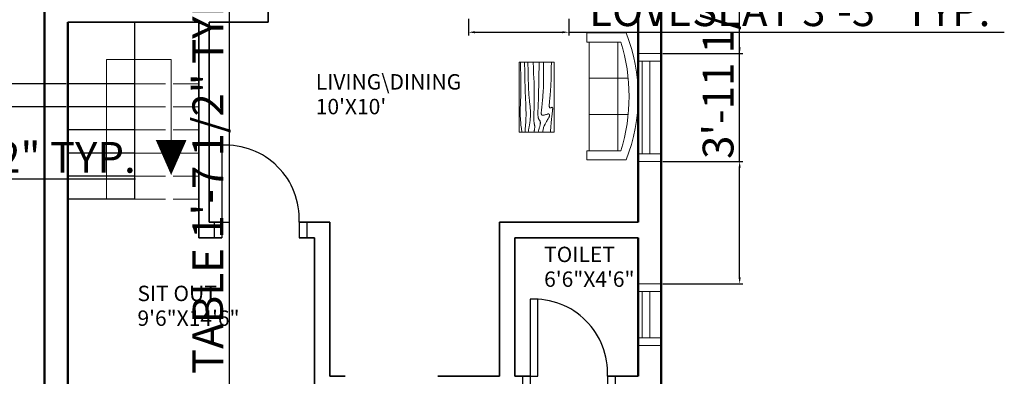
# Model space of a CAD drawing. Units: inches. Extents: x 2296 to 3335, y 495 to 1294.
# Tile 6 of 7: x 2952 to 3335, y 723 to 862. Entities that reach past the tile are written whole.
import ezdxf

# ---------------------------------------------------------------- set-up
doc = ezdxf.new("R2010")
doc.units = ezdxf.units.IN
doc.linetypes.add('ACAD_ISO02W100', pattern=[15, 12, -3])
for name, color, linetype, lineweight in [('A-ANNO-DIMS', 2, 'Continuous', 18), ('A-ANNO-SYMB', 7, 'Continuous', 18), ('A-AREA-IDEN', 7, 'Continuous', 18), ('A-FLOR-STRS', 7, 'Continuous', 25), ('A-FLOR-STRS-OVHD', 7, 'ACAD_ISO02W100', 18), ('DOORS', 1, 'Continuous', 25), ('FURNITURE', 2, 'Continuous', 18), ('INNER WALL', 6, 'Continuous', 35), ('OUTER WALL', 5, 'Continuous', 50), ('VENTILATOR', 4, 'Continuous', 18), ('WINDOWS', 3, 'Continuous', 18)]:
    doc.layers.add(name, color=color, linetype=linetype, lineweight=lineweight)
doc.styles.get("Standard").update_dxf_attribs({"font": 'arial.ttf'})
doc.dimstyles.new('ISO-25', dxfattribs={"dimtxt": 12, "dimasz": 2.5, "dimexe": 1.25, "dimexo": 0.625, "dimtad": 1, "dimdec": 1, "dimlunit": 3, "dimtxsty": 'Standard', "dimcen": 2.5, "dimadec": 0, "dimazin": 0, "dimtfac": 1, "dimtdec": 1, "dimtmove": 0, "dimatfit": 3, "dimfxl": 1, "dimarcsym": 0})

# ---------------------------------------------------------------- blocks, each defined once
blk = doc.blocks.new('Sofa - Roundback 7 ft.')
for p, q in [((-36.000027, -34), (-36.000027, -11.4696)), ((-12.00002, -32.4421), (-12.00003, -6.5971)), ((11.99997, -32.4421), (11.99998, -6.5971)), ((35.99998, -34), (35.99998, -11.4696)), ((-35.999844, -13.3819), (35.9998, -13.3819)), ((-36.000027, -32.4421), (35.99998, -32.4421))]:
    blk.add_line(p, q)
for points in [[(-36.000027, -34), (-42.000027, -34), (-42.000027, -8)], [(41.99998, -8), (41.99998, -34), (35.99998, -34)]]:
    blk.add_lwpolyline(points)
for centre, radius, start, end in [((0, -114.25), 114.25, 68.43141, 111.5686), ((-0.00001, -127.1968), 121.1968, 72.72033, 107.2797)]:
    blk.add_arc(centre, radius, start, end)
blk = doc.blocks.new('Table - Rectangular Woodgrain 60 x 30 in.')
for p, q in [((0, 0), (0, -30)), ((60, 0), (0, 0)), ((60, -30), (60, 0)), ((0, -30), (60, -30))]:
    blk.add_line(p, q)
for points in [[(0, -2.4), (4.8155, -2.418), (9.0302, -2.4688), (12.709, -2.5477), (15.9167, -2.65), (18.7181, -2.7711), (21.1781, -2.9063), (23.3616, -3.0508), (25.3333, -3.2), (27.1477, -3.3495), (28.8172, -3.4958), (30.3437, -3.636), (31.7291, -3.7667), (32.9756, -3.8849), (34.0849, -3.9875), (35.059, -4.0714), (35.9, -4.1334), (36.6114, -4.1711), (37.2041, -4.1854), (37.6906, -4.1779), (38.0833, -4.15), (38.3948, -4.1034), (38.6375, -4.0396), (38.8239, -3.9602), (38.9666, -3.8667), (39.0764, -3.7608), (39.1573, -3.6448), (39.2116, -3.521), (39.2416, -3.3917), (39.2498, -3.2593), (39.2385, -3.1261), (39.21, -2.9944), (39.1666, -2.8667), (39.111, -2.7447), (39.0468, -2.6281), (38.978, -2.5163), (38.9083, -2.4083), (38.8418, -2.3035), (38.7823, -2.201), (38.7337, -2.1001), (38.7, -2), (38.6844, -1.9003), (38.6875, -1.8021), (38.7094, -1.707), (38.75, -1.6167), (38.8094, -1.5326), (38.8875, -1.4563), (38.9844, -1.3893), (39.1, -1.3333), (39.2351, -1.2896), (39.3937, -1.2583), (39.5804, -1.2396), (39.8, -1.2333), (40.057, -1.2396), (40.3562, -1.2583), (40.7023, -1.2896), (41.1, -1.3333), (41.5547, -1.3895), (42.0755, -1.4573), (42.6721, -1.5361), (43.3542, -1.625), (44.1316, -1.7233), (45.014, -1.8302), (46.0114, -1.9449), (47.1333, -2.0667), (48.3862, -2.1947), (49.7625, -2.3281), (51.2513, -2.4663), (52.8416, -2.6083), (54.5226, -2.7535), (56.2833, -2.9011), (58.1127, -3.0501), (60, -3.2)], [(0, -9.2), (6.5759, -9.0858), (11.9385, -9.0365), (16.2527, -9.0418), (19.6833, -9.0917), (22.3952, -9.1759), (24.5531, -9.2844), (26.322, -9.4069), (27.8666, -9.5333), (29.3241, -9.6553), (30.7203, -9.7719), (32.0532, -9.8837), (33.3208, -9.9917), (34.5213, -10.0965), (35.6526, -10.199), (36.7128, -10.2999), (37.7, -10.4), (38.6129, -10.4996), (39.4531, -10.5969), (40.223, -10.6895), (40.925, -10.775), (41.5613, -10.8512), (42.1344, -10.9156), (42.6465, -10.966), (43.1, -11), (43.4976, -11.0158), (43.8437, -11.0136), (44.143, -10.9942), (44.4, -10.9583), (44.6195, -10.9069), (44.8062, -10.8406), (44.9648, -10.7603), (45.1, -10.6667), (45.2155, -10.5598), (45.3114, -10.4365), (45.3871, -10.2929), (45.4416, -10.125), (45.4743, -9.929), (45.4844, -9.7011), (45.4709, -9.4371), (45.4333, -9.1333), (45.3716, -8.7883), (45.2896, -8.4104), (45.1919, -8.0107), (45.0833, -7.6), (44.9685, -7.1893), (44.8521, -6.7896), (44.7388, -6.4117), (44.6333, -6.0667), (44.54, -5.7628), (44.4614, -5.4979), (44.4001, -5.2675), (44.3583, -5.0667), (44.3384, -4.8909), (44.3427, -4.7354), (44.3736, -4.5956), (44.4333, -4.4667), (44.5236, -4.3453), (44.6427, -4.2333), (44.7884, -4.1339), (44.9583, -4.05), (45.1501, -3.9849), (45.3614, -3.9417), (45.59, -3.9234), (45.8333, -3.9333), (46.0915, -3.9749), (46.3734, -4.0531), (46.6906, -4.1736), (47.0542, -4.3417), (47.4756, -4.5629), (47.9661, -4.8427), (48.5372, -5.1866), (49.2, -5.6), (49.9676, -6.0844), (50.8594, -6.625), (51.8965, -7.2031), (53.1, -7.8), (54.491, -8.3969), (56.0906, -8.975), (57.9199, -9.5156), (60, -10)], [(0, -12.8), (5.1847, -12.9322), (9.6213, -13.0323), (13.3963, -13.1059), (16.5958, -13.1583), (19.3063, -13.1952), (21.614, -13.2219), (23.6054, -13.2439), (25.3666, -13.2667), (26.9728, -13.2947), (28.4531, -13.3281), (29.8256, -13.3663), (31.1083, -13.4083), (32.3191, -13.4535), (33.476, -13.501), (34.597, -13.5501), (35.7, -13.6), (36.7984, -13.6497), (37.8875, -13.6979), (38.9578, -13.743), (40, -13.7833), (41.0047, -13.8174), (41.9625, -13.8438), (42.864, -13.8607), (43.7, -13.8667), (44.4631, -13.8604), (45.1552, -13.8417), (45.7801, -13.8104), (46.3416, -13.7667), (46.8439, -13.7104), (47.2906, -13.6417), (47.6858, -13.5604), (48.0333, -13.4667), (48.3375, -13.3608), (48.6042, -13.2448), (48.8396, -13.121), (49.05, -12.9917), (49.2417, -12.8593), (49.4208, -12.7261), (49.5937, -12.5944), (49.7667, -12.4667), (49.9452, -12.3451), (50.1323, -12.2313), (50.3303, -12.1268), (50.5416, -12.0333), (50.7686, -11.9524), (51.0135, -11.8854), (51.2788, -11.8341), (51.5666, -11.8), (51.8785, -11.7843), (52.2116, -11.7865), (52.562, -11.8059), (52.926, -11.8417), (53.2998, -11.8931), (53.6795, -11.9594), (54.0614, -12.0397), (54.4416, -12.1333), (54.8223, -12.2401), (55.2293, -12.3625), (55.6942, -12.5037), (56.2489, -12.6667), (56.9251, -12.8547), (57.7545, -13.0708), (58.7689, -13.3182), (60, -13.6)], [(0, -18), (5.124, -17.7273), (9.6609, -17.5057), (13.6705, -17.3303), (17.2125, -17.1958), (20.3467, -17.0973), (23.1328, -17.0297), (25.6307, -16.9878), (27.9, -16.9667), (29.9928, -16.9617), (31.9302, -16.9703), (33.7254, -16.9907), (35.3917, -17.0208), (36.9423, -17.0588), (38.3906, -17.1026), (39.7499, -17.1503), (41.0333, -17.2), (42.2519, -17.2496), (43.4073, -17.2969), (44.4986, -17.3395), (45.525, -17.375), (46.4858, -17.4012), (47.3802, -17.4156), (48.2074, -17.416), (48.9667, -17.4), (49.6583, -17.3662), (50.2872, -17.3167), (50.8595, -17.2547), (51.3812, -17.1833), (51.8584, -17.1057), (52.2971, -17.025), (52.7034, -16.9443), (53.0833, -16.8667), (53.443, -16.7951), (53.789, -16.7313), (54.128, -16.6768), (54.4666, -16.6334), (54.8115, -16.6024), (55.1693, -16.5854), (55.5465, -16.5841), (55.95, -16.6), (56.3828, -16.6337), (56.8346, -16.6823), (57.2915, -16.7418), (57.7396, -16.8084), (58.165, -16.878), (58.5539, -16.9469), (58.8924, -17.0111), (59.1666, -17.0667), (59.3679, -17.1107), (59.5078, -17.1438), (59.6032, -17.1675), (59.6708, -17.1833), (59.7275, -17.193), (59.7901, -17.1979), (59.8753, -17.1998), (60, -17.2)], [(0, -22.4), (8.0098, -22.2501), (14.4094, -22.1011), (19.4168, -21.9535), (23.25, -21.8083), (26.1269, -21.6663), (28.2656, -21.5281), (29.884, -21.3947), (31.2, -21.2667), (32.3967, -21.1448), (33.5172, -21.0292), (34.5697, -20.9198), (35.5625, -20.8167), (36.5037, -20.7198), (37.4015, -20.6292), (38.2642, -20.5448), (39.1, -20.4667), (39.9164, -20.3951), (40.7187, -20.3313), (41.5117, -20.2768), (42.3, -20.2333), (43.0883, -20.2024), (43.8812, -20.1854), (44.6836, -20.1841), (45.5, -20.2), (46.3328, -20.234), (47.1747, -20.2844), (48.0163, -20.3488), (48.8479, -20.425), (49.66, -20.5106), (50.4429, -20.6031), (51.1872, -20.7004), (51.8833, -20.8), (52.5246, -20.8999), (53.1166, -20.9995), (53.6681, -21.0983), (54.1875, -21.1958), (54.6834, -21.2919), (55.1646, -21.3859), (55.6394, -21.4777), (56.1167, -21.5667), (56.6028, -21.6515), (57.0961, -21.7266), (57.5929, -21.7852), (58.0896, -21.8208), (58.5823, -21.8268), (59.0674, -21.7964), (59.5412, -21.723), (60, -21.6)], [(0, -25.2), (8.6355, -25.0504), (15.7026, -24.9031), (21.4049, -24.7606), (25.9458, -24.625), (29.529, -24.4988), (32.3578, -24.3844), (34.6359, -24.284), (36.5667, -24.2), (38.3213, -24.1341), (39.9417, -24.0854), (41.437, -24.0523), (42.8167, -24.0333), (44.0901, -24.0268), (45.2667, -24.0313), (46.3557, -24.0451), (47.3667, -24.0667), (48.309, -24.0947), (49.1928, -24.1287), (50.0284, -24.168), (50.826, -24.2125), (51.5959, -24.2617), (52.3483, -24.3151), (53.0935, -24.3725), (53.8417, -24.4334), (54.6009, -24.497), (55.3699, -24.561), (56.1454, -24.6226), (56.9239, -24.6792), (57.7021, -24.7279), (58.4764, -24.7662), (59.2435, -24.7911), (60, -24.8)], [(0, -28.8), (5.6867, -28.6681), (10.45, -28.5698), (14.407, -28.5012), (17.675, -28.4584), (20.3711, -28.4374), (22.6125, -28.4344), (24.5164, -28.4455), (26.2, -28.4667), (27.762, -28.4947), (29.2276, -28.5281), (30.6033, -28.5663), (31.8958, -28.6084), (33.1118, -28.6535), (34.2578, -28.7011), (35.3405, -28.7501), (36.3666, -28.8), (37.3443, -28.8497), (38.288, -28.8974), (39.2137, -28.9412), (40.1375, -28.9792), (41.0753, -29.0093), (42.0432, -29.0297), (43.0572, -29.0384), (44.1333, -29.0333), (45.2936, -29.0114), (46.5843, -28.9641), (48.0579, -28.8816), (49.7666, -28.7542), (51.7629, -28.5721), (54.0989, -28.3255), (56.8272, -28.0048), (60, -27.6)]]:
    blk.add_lwpolyline(points)
blk = doc.blocks.new('DOOR-SINGLE-30IN')
for p, q in [((-3, 0), (-3, -6)), ((0, 0), (0, -6)), ((30, 0), (30, -6)), ((33, 0), (33, -6))]:
    blk.add_line(p, q)
blk.add_lwpolyline([(0, 0), (3, 0), (3, 30), (0, 30)], close=True)
blk.add_arc((1.5, 1.5), 28.54, 356.9872, 93.0128)
blk = doc.blocks.new('WIN-36IN')
for p, q in [((0, 42), (9, 42)), ((0, 39), (9, 39)), ((1.5, 3), (1.5, 39)), ((4.5, 3), (4.5, 39)), ((9, 3), (0, 3)), ((9, 0), (0, 0))]:
    blk.add_line(p, q)
blk = doc.blocks.new('VENT-18IN')
for p, q in [((0, 24), (9, 24)), ((0, 21), (9, 21)), ((4.5, 21), (4.5, 3)), ((7.5, 21), (7.5, 3)), ((9, 3), (0, 3)), ((9, 0), (0, 0))]:
    blk.add_line(p, q)
blk = doc.blocks.new('*D41')
at = {"layer": 'A-ANNO-DIMS', "color": 0, "lineweight": -2, "transparency": 16777216}
for p, q in [((3126.63, 862.3), (3126.63, 855.82)), ((3165.62, 862.3), (3165.62, 855.82)), ((3129.13, 857.07), (3163.12, 857.07)), ((3165.62, 857.07), (3335.15, 857.07))]:
    blk.add_line(p, q, dxfattribs=at)
at = {"layer": 'A-ANNO-DIMS', "color": 0, "transparency": 16777216}
for points in [[(3129.13, 857.49), (3129.13, 856.66), (3126.63, 857.07)], [(3163.12, 857.49), (3163.12, 856.66), (3165.62, 857.07)]]:
    blk.add_solid(points, dxfattribs=at)
at = {"layer": 'Defpoints', "color": 0, "transparency": 16777216}
for p in [(3126.63, 862.92), (3165.62, 862.92), (3165.62, 857.07)]:
    blk.add_point(p, dxfattribs=at)
at = {"layer": 'A-ANNO-DIMS', "color": 0, "transparency": 16777216, "insert": (3251.64, 863.91), "char_height": 12, "attachment_point": 5}
blk.add_mtext('LOVESEAT 3\'-3" TYP.', dxfattribs=at)
blk = doc.blocks.new('*D44')
at = {"layer": 'A-ANNO-DIMS', "color": 0, "lineweight": -2, "transparency": 16777216}
for p, q in [((2871.66, 806.74), (2871.66, 798.71)), ((2893.23, 806.74), (2893.23, 798.71)), ((2874.16, 799.96), (2890.73, 799.96)), ((2893.23, 799.96), (2996.95, 799.96))]:
    blk.add_line(p, q, dxfattribs=at)
at = {"layer": 'A-ANNO-DIMS', "color": 0, "transparency": 16777216}
for points in [[(2874.16, 800.37), (2874.16, 799.54), (2871.66, 799.96)], [(2890.73, 800.37), (2890.73, 799.54), (2893.23, 799.96)]]:
    blk.add_solid(points, dxfattribs=at)
at = {"layer": 'Defpoints', "color": 0, "transparency": 16777216}
for p in [(2871.66, 807.37), (2893.23, 807.37), (2893.23, 799.96)]:
    blk.add_point(p, dxfattribs=at)
at = {"layer": 'A-ANNO-DIMS', "color": 0, "transparency": 16777216, "insert": (2946.34, 806.78), "char_height": 12, "attachment_point": 5}
blk.add_mtext('1\'-9 1/2" TYP.', dxfattribs=at)
blk = doc.blocks.new('*D49')
at = {"layer": 'A-ANNO-DIMS', "color": 0, "lineweight": -2, "transparency": 16777216}
for p, q in [((3033.55, 677.03), (3033.55, 883.38)), ((3031.26, 677.03), (3034.8, 677.03)), ((3033.55, 660.07), (3033.55, 674.53)), ((3031.26, 657.57), (3034.8, 657.57))]:
    blk.add_line(p, q, dxfattribs=at)
at = {"layer": 'A-ANNO-DIMS', "color": 0, "transparency": 16777216}
for points in [[(3033.13, 674.53), (3033.97, 674.53), (3033.55, 677.03)], [(3033.13, 660.07), (3033.97, 660.07), (3033.55, 657.57)]]:
    blk.add_solid(points, dxfattribs=at)
at = {"layer": 'Defpoints', "color": 0, "transparency": 16777216}
for p in [(3030.63, 677.03), (3033.55, 677.03), (3030.63, 657.57)]:
    blk.add_point(p, dxfattribs=at)
at = {"layer": 'A-ANNO-DIMS', "color": 0, "transparency": 16777216, "insert": (3026.72, 781.45), "char_height": 12, "attachment_point": 5, "rotation": 90}
blk.add_mtext('SIDE TABLE 1\'-7 1/2" TYP.', dxfattribs=at)
blk = doc.blocks.new('*D54')
at = {"layer": 'A-ANNO-DIMS', "color": 0, "lineweight": -2, "transparency": 16777216}
for p, q in [((2961.02, 1068.02), (2929.9, 1068.02)), ((2931.15, 590.52), (2931.15, 1065.52)), ((2961.02, 588.02), (2929.9, 588.02))]:
    blk.add_line(p, q, dxfattribs=at)
at = {"layer": 'A-ANNO-DIMS', "color": 0, "transparency": 16777216}
for points in [[(2930.73, 1065.52), (2931.56, 1065.52), (2931.15, 1068.02)], [(2930.73, 590.52), (2931.56, 590.52), (2931.15, 588.02)]]:
    blk.add_solid(points, dxfattribs=at)
at = {"layer": 'Defpoints', "color": 0, "transparency": 16777216}
for p in [(2931.15, 1068.02), (2961.65, 1068.02), (2961.65, 588.02)]:
    blk.add_point(p, dxfattribs=at)
at = {"layer": 'A-ANNO-DIMS', "color": 0, "transparency": 16777216, "insert": (2924.39, 828.02), "char_height": 12, "attachment_point": 5, "rotation": 90}
blk.add_mtext('40\'-0"', dxfattribs=at)
blk = doc.blocks.new('*D66')
at = {"layer": 'A-ANNO-DIMS', "color": 0, "lineweight": -2, "transparency": 16777216}
for p, q in [((2931.15, 837.02), (2931.15, 872.67)), ((2970.02, 837.02), (2929.9, 837.02)), ((2931.15, 830.52), (2931.15, 834.52)), ((2970.02, 828.02), (2929.9, 828.02))]:
    blk.add_line(p, q, dxfattribs=at)
at = {"layer": 'A-ANNO-DIMS', "color": 0, "transparency": 16777216}
for points in [[(2930.73, 834.52), (2931.56, 834.52), (2931.15, 837.02)], [(2930.73, 830.52), (2931.56, 830.52), (2931.15, 828.02)]]:
    blk.add_solid(points, dxfattribs=at)
at = {"layer": 'Defpoints', "color": 0, "transparency": 16777216}
for p in [(2931.15, 837.02), (2970.65, 837.02), (2970.65, 828.02)]:
    blk.add_point(p, dxfattribs=at)
at = {"layer": 'A-ANNO-DIMS', "color": 0, "transparency": 16777216, "insert": (2924.39, 856.09), "char_height": 12, "attachment_point": 5, "rotation": 90}
blk.add_mtext('0\'-9"', dxfattribs=at)
blk = doc.blocks.new('*D74')
at = {"layer": 'A-ANNO-DIMS', "color": 0, "lineweight": -2, "transparency": 16777216}
for p, q in [((3202.27, 948.82), (3233.4, 948.82)), ((3232.15, 851.25), (3232.15, 946.32)), ((3202.27, 848.75), (3233.4, 848.75))]:
    blk.add_line(p, q, dxfattribs=at)
at = {"layer": 'A-ANNO-DIMS', "color": 0, "transparency": 16777216}
for points in [[(3231.73, 946.32), (3232.56, 946.32), (3232.15, 948.82)], [(3231.73, 851.25), (3232.56, 851.25), (3232.15, 848.75)]]:
    blk.add_solid(points, dxfattribs=at)
at = {"layer": 'Defpoints', "color": 0, "transparency": 16777216}
for p in [(3201.65, 948.82), (3232.15, 948.82), (3201.65, 848.75)]:
    blk.add_point(p, dxfattribs=at)
at = {"layer": 'A-ANNO-DIMS', "color": 0, "transparency": 16777216, "insert": (3225.39, 898.79), "char_height": 12, "attachment_point": 5, "rotation": 90}
blk.add_mtext('8\'-4"', dxfattribs=at)
blk = doc.blocks.new('*D75')
at = {"layer": 'A-ANNO-DIMS', "color": 0, "lineweight": -2, "transparency": 16777216}
for p, q in [((3232.15, 806.75), (3232.15, 879.68)), ((3202.27, 806.75), (3233.4, 806.75)), ((3232.15, 761.57), (3232.15, 804.25)), ((3202.27, 759.07), (3233.4, 759.07))]:
    blk.add_line(p, q, dxfattribs=at)
at = {"layer": 'A-ANNO-DIMS', "color": 0, "transparency": 16777216}
for points in [[(3231.73, 804.25), (3232.56, 804.25), (3232.15, 806.75)], [(3231.73, 761.57), (3232.56, 761.57), (3232.15, 759.07)]]:
    blk.add_solid(points, dxfattribs=at)
at = {"layer": 'Defpoints', "color": 0, "transparency": 16777216}
for p in [(3201.65, 806.75), (3232.15, 806.75), (3201.65, 759.07)]:
    blk.add_point(p, dxfattribs=at)
at = {"layer": 'A-ANNO-DIMS', "color": 0, "transparency": 16777216, "insert": (3225.31, 844.47), "char_height": 12, "attachment_point": 5, "rotation": 90}
blk.add_mtext('3\'-11 1/2"', dxfattribs=at)

msp = doc.modelspace()

# ---------------------------------------------------------------- linework, layer by layer
at = {"layer": 'A-ANNO-SYMB'}
msp.add_lwpolyline([(3010.88, 815.12), (3010.88, 846.46), (2985.68, 846.46), (2985.68, 792.02)], dxfattribs=at)
msp.add_lwpolyline([(3010.88, 815.12, 12, 0, 0), (3010.88, 801.45, 0, 0, 0)], format="xyseb", dxfattribs=at)
at = {"layer": 'A-FLOR-STRS'}
for p, q in [((2996.65, 861.02), (2996.65, 792.02)), ((2996.65, 837.02), (2970.65, 837.02)), ((2996.65, 828.02), (2970.65, 828.02)), ((2996.65, 819.02), (2970.65, 819.02)), ((2996.65, 810.02), (2970.65, 810.02)), ((2996.65, 801.02), (2970.65, 801.02)), ((2996.65, 792.02), (2970.65, 792.02))]:
    msp.add_line(p, q, dxfattribs=at)
at = {"layer": 'A-FLOR-STRS-OVHD'}
for p, q in [((2996.65, 837.02), (3021.65, 837.02)), ((2996.65, 828.02), (3021.65, 828.02)), ((2996.65, 819.02), (3021.65, 819.02)), ((2996.65, 810.02), (3021.65, 810.02)), ((2996.65, 801.02), (3021.65, 801.02)), ((2996.65, 792.02), (3021.65, 792.02))]:
    msp.add_line(p, q, dxfattribs=at)
at = {"layer": 'INNER WALL'}
for p, q in [((3048.65, 915.02), (3048.65, 861.02)), ((3021.65, 861.02), (2970.65, 861.02)), ((3021.65, 861.02), (3021.65, 777.02)), ((3048.65, 861.02), (3025.65, 861.02)), ((3025.65, 861.02), (3025.65, 783.02)), ((3025.65, 783.02), (3030.65, 783.02)), ((3060.65, 783.02), (3072.65, 783.02)), ((3072.65, 723.02), (3072.65, 783.02)), ((3138.65, 783.02), (3192.65, 783.02)), ((3138.65, 723.02), (3138.65, 783.02)), ((3021.65, 777.02), (3030.65, 777.02)), ((3060.65, 777.02), (3066.65, 777.02)), ((3066.65, 588.02), (3066.65, 777.02)), ((3144.65, 777.02), (3192.65, 777.02)), ((3144.65, 723.02), (3144.65, 777.02)), ((3072.65, 723.02), (3078.65, 723.02)), ((3114.65, 723.02), (3138.65, 723.02)), ((3144.65, 723.02), (3150.65, 723.02)), ((3180.65, 723.02), (3192.65, 723.02))]:
    msp.add_line(p, q, dxfattribs=at)
at = {"layer": 'OUTER WALL'}
for p, q in [((3192.65, 783.02), (3192.65, 885.02)), ((2970.65, 861.02), (2970.65, 588.02)), ((3192.65, 723.02), (3192.65, 777.02))]:
    msp.add_line(p, q, dxfattribs=at)
msp.add_lwpolyline([(3066.65, 588.02), (3201.65, 588.02), (3201.65, 1068.02), (2961.65, 1068.02), (2961.65, 588.02), (2970.65, 588.02)], dxfattribs=at)

# ---------------------------------------------------------------- block references
at = {"layer": 'DOORS'}
for p in [(3030.65, 783.02), (3150.65, 723.02)]:
    msp.add_blockref('DOOR-SINGLE-30IN', p, dxfattribs=at)
at = {"layer": 'FURNITURE', "rotation": 270}
for name, p, xscale, yscale, zscale in [('Sofa - Roundback 7 ft.', (3192.65, 832.08), 0.588291610216848, 0.588291610216848, 0.588291610216848), ('Table - Rectangular Woodgrain 60 x 30 in.', (3159.95, 845.46), 0.455660307090303, 0.455660307090303, 0.455660307090303)]:
    msp.add_blockref(name, p, dxfattribs=dict(at, xscale=xscale, yscale=yscale, zscale=zscale))
at = {"layer": 'VENTILATOR', "rotation": 180}
msp.add_blockref('VENT-18IN', (3201.65, 759.07), dxfattribs=at)
at = {"layer": 'WINDOWS'}
msp.add_blockref('WIN-36IN', (3192.65, 806.75), dxfattribs=at)

# ---------------------------------------------------------------- texts
at = {"layer": 'A-AREA-IDEN'}
for s, p in [('LIVING\\DINING', (3067.16, 834.74)), ("10'X10'", (3067.16, 825.11)), ('TOILET', (3156.04, 767.52)), ('6\'6"X4\'6"', (3156.04, 757.88)), ('SIT OUT', (2997.77, 752.32)), ('9\'6"X14\'6"', (2997.77, 742.68))]:
    msp.add_text(s, height=6, dxfattribs=at).set_placement(p)

# ---------------------------------------------------------------- dimensions: what is measured, and where the dimension line sits
at = {"layer": 'A-ANNO-DIMS'}
for base, p1, p2, picture, middle in [((2931.15, 1068.02), (2961.65, 588.02), (2961.65, 1068.02), '*D54', (2924.39, 828.02)), ((3232.15, 948.82), (3201.65, 848.75), (3201.65, 948.82), '*D74', (3225.39, 898.79)), ((3232.15, 806.75), (3201.65, 759.07), (3201.65, 806.75), '*D75', (3225.31, 844.47)), ((2931.15, 837.02), (2970.65, 828.02), (2970.65, 837.02), '*D66', (2924.39, 856.09))]:
    dim = msp.add_linear_dim(base=base, p1=p1, p2=p2, angle=90, dimstyle='ISO-25', override={"dimdec": 1, "dimlfac": 1, "dimrnd": 0, "dimzin": 1, "dimdsep": 46, "dimlunit": 4, "dimfrac": 2}, dxfattribs=at)
    dim.commit()
    dim.dimension.update_dxf_attribs({"geometry": picture, "text_midpoint": middle})
for base, p1, p2, text, picture, middle in [((3165.62, 857.07), (3126.63, 862.92), (3165.62, 862.92), 'LOVESEAT <> TYP.', '*D41', (3251.64, 863.91)), ((2893.23, 799.96), (2871.66, 807.37), (2893.23, 807.37), '<> TYP.', '*D44', (2946.34, 806.78))]:
    dim = msp.add_linear_dim(base=base, p1=p1, p2=p2, text=text, dimstyle='ISO-25', override={"dimdec": 1, "dimlfac": 1, "dimrnd": 0, "dimzin": 1, "dimdsep": 46, "dimlunit": 4, "dimfrac": 2}, dxfattribs=at)
    dim.commit()
    dim.dimension.update_dxf_attribs({"geometry": picture, "text_midpoint": middle})
dim = msp.add_linear_dim(base=(3033.55, 677.03), p1=(3030.63, 657.57), p2=(3030.63, 677.03), angle=90, text='SIDE TABLE <> TYP.', dimstyle='ISO-25', override={"dimdec": 1, "dimlfac": 1, "dimrnd": 0, "dimzin": 1, "dimdsep": 46, "dimlunit": 4, "dimfrac": 2}, dxfattribs=at)
dim.commit()
dim.dimension.update_dxf_attribs({"geometry": '*D49', "text_midpoint": (3026.72, 781.45)})

doc.saveas('drawing.dxf')
